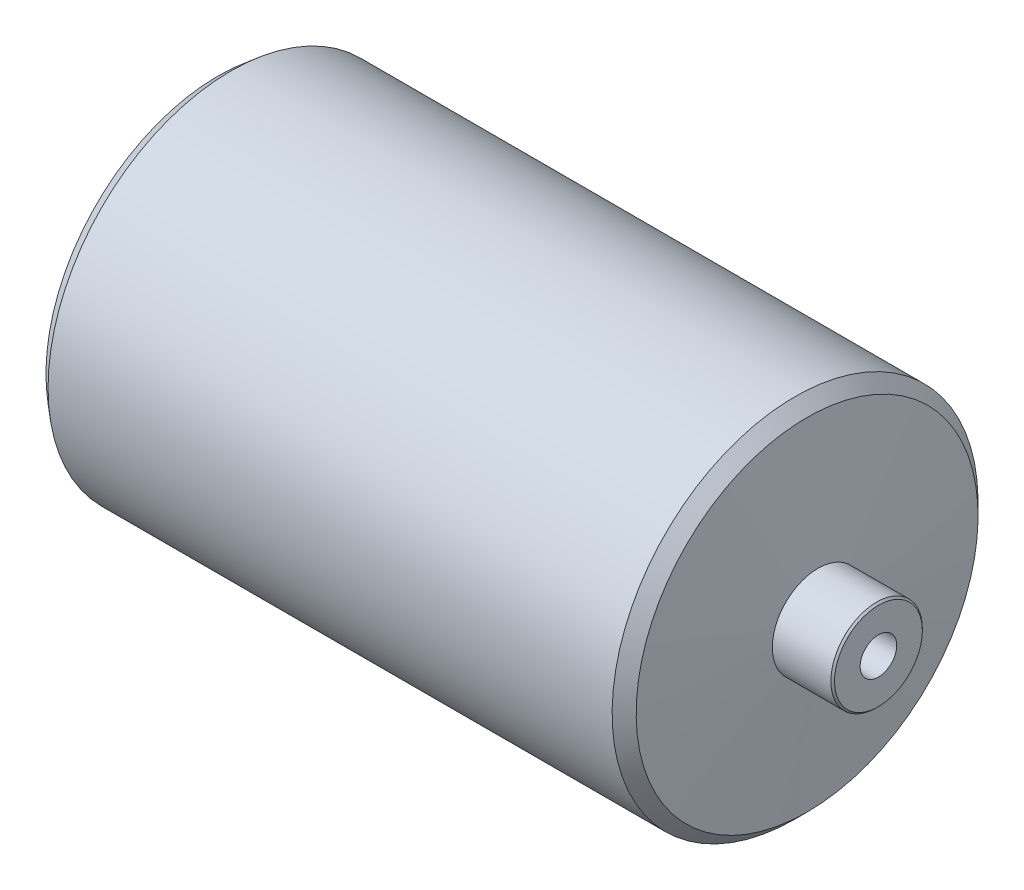
ISO-10303-21;
HEADER;
FILE_DESCRIPTION(('STEP AP214'),'2;1');
FILE_NAME('part.step','',(''),(''),'','','');
FILE_SCHEMA(('AUTOMOTIVE_DESIGN { 1 0 10303 214 1 1 1 1 }'));
ENDSEC;
DATA;
#1=APPLICATION_CONTEXT('core data for automotive mechanical design processes');
#2=APPLICATION_PROTOCOL_DEFINITION('international standard','automotive_design',2000,#1);
#3=PRODUCT_CONTEXT('',#1,'mechanical');
#4=PRODUCT('Part','Part','',(#3));
#5=PRODUCT_RELATED_PRODUCT_CATEGORY('part','',(#4));
#6=PRODUCT_DEFINITION_FORMATION('','',#4);
#7=PRODUCT_DEFINITION_CONTEXT('part definition',#1,'design');
#8=PRODUCT_DEFINITION('design','',#6,#7);
#9=PRODUCT_DEFINITION_SHAPE('','',#8);
#10=(LENGTH_UNIT() NAMED_UNIT(*) SI_UNIT(.MILLI.,.METRE.));
#11=(NAMED_UNIT(*) PLANE_ANGLE_UNIT() SI_UNIT($,.RADIAN.));
#12=(NAMED_UNIT(*) SI_UNIT($,.STERADIAN.) SOLID_ANGLE_UNIT());
#13=UNCERTAINTY_MEASURE_WITH_UNIT(LENGTH_MEASURE(1.E-05),#10,'distance_accuracy_value','');
#14=(GEOMETRIC_REPRESENTATION_CONTEXT(3) GLOBAL_UNCERTAINTY_ASSIGNED_CONTEXT((#13)) GLOBAL_UNIT_ASSIGNED_CONTEXT((#10,
#11,#12)) REPRESENTATION_CONTEXT('',''));
#15=CARTESIAN_POINT('',(0.,0.,0.));
#16=DIRECTION('',(0.,0.,1.));
#17=DIRECTION('',(1.,0.,0.));
#18=AXIS2_PLACEMENT_3D('',#15,#16,#17);
#19=CARTESIAN_POINT('',(0.,0.,0.));
#20=DIRECTION('',(-1.,0.,0.));
#21=DIRECTION('',(0.,-1.,0.));
#22=AXIS2_PLACEMENT_3D('',#19,#20,#21);
#23=PLANE('',#22);
#24=CARTESIAN_POINT('',(0.,0.,0.));
#25=DIRECTION('',(-1.,0.,0.));
#26=DIRECTION('',(0.,0.,1.));
#27=AXIS2_PLACEMENT_3D('',#24,#25,#26);
#28=CIRCLE('',#27,5.00000000000001);
#29=CARTESIAN_POINT('',(0.,0.,5.00000000000001));
#30=VERTEX_POINT('',#29);
#31=EDGE_CURVE('E90',#30,#30,#28,.T.);
#32=ORIENTED_EDGE('',*,*,#31,.F.);
#33=EDGE_LOOP('',(#32));
#34=FACE_BOUND('',#33,.T.);
#35=CARTESIAN_POINT('',(0.,0.,0.));
#36=DIRECTION('',(-1.,0.,0.));
#37=DIRECTION('',(0.,-1.,0.));
#38=AXIS2_PLACEMENT_3D('',#35,#36,#37);
#39=CIRCLE('',#38,12.);
#40=CARTESIAN_POINT('',(0.,-12.,0.));
#41=VERTEX_POINT('',#40);
#42=EDGE_CURVE('E58',#41,#41,#39,.T.);
#43=ORIENTED_EDGE('',*,*,#42,.T.);
#44=EDGE_LOOP('',(#43));
#45=FACE_BOUND('',#44,.T.);
#46=ADVANCED_FACE('F39',(#34,#45),#23,.T.);
#47=CARTESIAN_POINT('',(200.,0.,0.));
#48=DIRECTION('',(1.,0.,0.));
#49=DIRECTION('',(0.,1.,0.));
#50=AXIS2_PLACEMENT_3D('',#47,#48,#49);
#51=CYLINDRICAL_SURFACE('',#50,12.5);
#52=CARTESIAN_POINT('',(0.500000000000056,0.,0.));
#53=DIRECTION('',(-1.,0.,0.));
#54=DIRECTION('',(0.,-1.,0.));
#55=AXIS2_PLACEMENT_3D('',#52,#53,#54);
#56=CIRCLE('',#55,12.5);
#57=CARTESIAN_POINT('',(0.500000000000057,-12.5,0.));
#58=VERTEX_POINT('',#57);
#59=EDGE_CURVE('E62',#58,#58,#56,.F.);
#60=ORIENTED_EDGE('',*,*,#59,.T.);
#61=EDGE_LOOP('',(#60));
#62=FACE_BOUND('',#61,.T.);
#63=CARTESIAN_POINT('',(16.5,0.,0.));
#64=DIRECTION('',(1.,0.,0.));
#65=DIRECTION('',(0.,1.,0.));
#66=AXIS2_PLACEMENT_3D('',#63,#64,#65);
#67=CIRCLE('',#66,12.5);
#68=CARTESIAN_POINT('',(16.5,12.5,0.));
#69=VERTEX_POINT('',#68);
#70=EDGE_CURVE('E75',#69,#69,#67,.T.);
#71=ORIENTED_EDGE('',*,*,#70,.F.);
#72=EDGE_LOOP('',(#71));
#73=FACE_BOUND('',#72,.T.);
#74=ADVANCED_FACE('F94',(#62,#73),#51,.T.);
#75=CARTESIAN_POINT('',(19.7808248822223,0.,0.));
#76=DIRECTION('',(1.,0.,0.));
#77=DIRECTION('',(0.,1.,0.));
#78=AXIS2_PLACEMENT_3D('',#75,#76,#77);
#79=CONICAL_SURFACE('',#78,50.,1.48352986419518);
#80=CARTESIAN_POINT('',(19.5193576539793,0.,0.));
#81=DIRECTION('',(-1.,0.,0.));
#82=DIRECTION('',(0.,-1.,0.));
#83=AXIS2_PLACEMENT_3D('',#80,#81,#82);
#84=CIRCLE('',#83,47.0114159057247);
#85=CARTESIAN_POINT('',(19.5193576539793,47.0114159057247,0.));
#86=VERTEX_POINT('',#85);
#87=EDGE_CURVE('E50',#86,#86,#84,.T.);
#88=CARTESIAN_POINT('',(19.5193576539793,47.0114159057247,0.));
#89=CARTESIAN_POINT('',(19.4879060117504,46.6519219900401,0.));
#90=CARTESIAN_POINT('',(19.4564543695214,46.2924280743555,0.));
#91=CARTESIAN_POINT('',(19.3935510850635,45.5734402429862,0.));
#92=CARTESIAN_POINT('',(19.3620994428346,45.2139463273016,0.));
#93=CARTESIAN_POINT('',(19.2991961583767,44.4949584959323,0.));
#94=CARTESIAN_POINT('',(19.2677445161477,44.1354645802477,0.));
#95=CARTESIAN_POINT('',(19.2048412316898,43.4164767488784,0.));
#96=CARTESIAN_POINT('',(19.1733895894609,43.0569828331938,0.));
#97=CARTESIAN_POINT('',(19.1104863050029,42.3379950018245,0.));
#98=CARTESIAN_POINT('',(19.079034662774,41.9785010861399,0.));
#99=CARTESIAN_POINT('',(19.0161313783161,41.2595132547706,0.));
#100=CARTESIAN_POINT('',(18.9846797360871,40.900019339086,0.));
#101=CARTESIAN_POINT('',(18.9217764516292,40.1810315077167,0.));
#102=CARTESIAN_POINT('',(18.8903248094003,39.8215375920321,0.));
#103=CARTESIAN_POINT('',(18.8274215249424,39.1025497606628,0.));
#104=CARTESIAN_POINT('',(18.7959698827134,38.7430558449782,0.));
#105=CARTESIAN_POINT('',(18.7330665982555,38.0240680136089,0.));
#106=CARTESIAN_POINT('',(18.7016149560266,37.6645740979243,0.));
#107=CARTESIAN_POINT('',(18.6387116715687,36.945586266555,0.));
#108=CARTESIAN_POINT('',(18.6072600293397,36.5860923508704,0.));
#109=CARTESIAN_POINT('',(18.5443567448818,35.8671045195011,0.));
#110=CARTESIAN_POINT('',(18.5129051026529,35.5076106038165,0.));
#111=CARTESIAN_POINT('',(18.450001818195,34.7886227724472,0.));
#112=CARTESIAN_POINT('',(18.418550175966,34.4291288567626,0.));
#113=CARTESIAN_POINT('',(18.3556468915081,33.7101410253933,0.));
#114=CARTESIAN_POINT('',(18.3241952492792,33.3506471097087,0.));
#115=CARTESIAN_POINT('',(18.2612919648213,32.6316592783394,0.));
#116=CARTESIAN_POINT('',(18.2298403225923,32.2721653626548,0.));
#117=CARTESIAN_POINT('',(18.1669370381344,31.5531775312855,0.));
#118=CARTESIAN_POINT('',(18.1354853959055,31.1936836156009,0.));
#119=CARTESIAN_POINT('',(18.0725821114476,30.4746957842316,0.));
#120=CARTESIAN_POINT('',(18.0411304692186,30.115201868547,0.));
#121=CARTESIAN_POINT('',(17.9782271847607,29.3962140371777,0.));
#122=CARTESIAN_POINT('',(17.9467755425318,29.0367201214931,0.));
#123=CARTESIAN_POINT('',(17.8838722580739,28.3177322901238,0.));
#124=CARTESIAN_POINT('',(17.8524206158449,27.9582383744392,0.));
#125=CARTESIAN_POINT('',(17.789517331387,27.2392505430699,0.));
#126=CARTESIAN_POINT('',(17.7580656891581,26.8797566273853,0.));
#127=CARTESIAN_POINT('',(17.6951624047002,26.160768796016,0.));
#128=CARTESIAN_POINT('',(17.6637107624712,25.8012748803314,0.));
#129=CARTESIAN_POINT('',(17.6008074780133,25.0822870489621,0.));
#130=CARTESIAN_POINT('',(17.5693558357844,24.7227931332775,0.));
#131=CARTESIAN_POINT('',(17.5064525513264,24.0038053019082,0.));
#132=CARTESIAN_POINT('',(17.4750009090975,23.6443113862236,0.));
#133=CARTESIAN_POINT('',(17.4120976246396,22.9253235548543,0.));
#134=CARTESIAN_POINT('',(17.3806459824106,22.5658296391697,0.));
#135=CARTESIAN_POINT('',(17.3177426979527,21.8468418078004,0.));
#136=CARTESIAN_POINT('',(17.2862910557238,21.4873478921158,0.));
#137=CARTESIAN_POINT('',(17.2233877712659,20.7683600607465,0.));
#138=CARTESIAN_POINT('',(17.1919361290369,20.4088661450619,0.));
#139=CARTESIAN_POINT('',(17.129032844579,19.6898783136926,0.));
#140=CARTESIAN_POINT('',(17.0975812023501,19.330384398008,0.));
#141=CARTESIAN_POINT('',(17.0346779178922,18.6113965666387,0.));
#142=CARTESIAN_POINT('',(17.0032262756632,18.2519026509541,0.));
#143=CARTESIAN_POINT('',(16.9403229912053,17.5329148195848,0.));
#144=CARTESIAN_POINT('',(16.9088713489764,17.1734209039002,0.));
#145=CARTESIAN_POINT('',(16.8459680645185,16.4544330725309,0.));
#146=CARTESIAN_POINT('',(16.8145164222895,16.0949391568463,0.));
#147=CARTESIAN_POINT('',(16.7516131378316,15.375951325477,0.));
#148=CARTESIAN_POINT('',(16.7201614956027,15.0164574097924,0.));
#149=CARTESIAN_POINT('',(16.6572582111448,14.2974695784231,0.));
#150=CARTESIAN_POINT('',(16.6258065689158,13.9379756627385,0.));
#151=CARTESIAN_POINT('',(16.5629032844579,13.2189878313692,0.));
#152=CARTESIAN_POINT('',(16.531451642229,12.8594939156846,0.));
#153=CARTESIAN_POINT('',(16.5,12.5,0.));
#154=B_SPLINE_CURVE_WITH_KNOTS('',3,(#88,#89,#90,#91,#92,#93,#94,#95,#96,#97,#98,#99,#100,#101,
#102,#103,#104,#105,#106,#107,#108,#109,#110,#111,#112,#113,#114,#115,#116,#117,#118,#119,#120,
#121,#122,#123,#124,#125,#126,#127,#128,#129,#130,#131,#132,#133,#134,#135,#136,#137,#138,#139,
#140,#141,#142,#143,#144,#145,#146,#147,#148,#149,#150,#151,#152,#153),.UNSPECIFIED.,.F.,.F.,(4,
2,2,2,2,2,2,2,2,2,2,2,2,2,2,2,2,2,2,2,2,2,2,2,2,2,2,2,2,2,2,2,4),(0.,1.08260137212111,
2.16520274424222,3.24780411636333,4.33040548848443,5.41300686060555,6.49560823272666,
7.57820960484777,8.66081097696888,9.74341234908999,10.8260137212111,11.9086150933322,
12.9912164654533,14.0738178375744,15.1564192096955,16.2390205818167,17.3216219539378,
18.4042233260589,19.48682469818,20.5694260703011,21.6520274424222,22.7346288145433,
23.8172301866644,24.8998315587855,25.9824329309067,27.0650343030278,28.1476356751489,
29.23023704727,30.3128384193911,31.3954397915122,32.4780411636333,33.5606425357544,
34.6432439078755),.UNSPECIFIED.);
#155=EDGE_CURVE('BSEAM107',#86,#69,#154,.T.);
#156=ORIENTED_EDGE('',*,*,#87,.T.);
#157=ORIENTED_EDGE('',*,*,#70,.T.);
#158=ORIENTED_EDGE('',*,*,#155,.T.);
#159=ORIENTED_EDGE('',*,*,#155,.F.);
#160=EDGE_LOOP('',(#156,#158,#157,#159));
#161=FACE_BOUND('',#160,.T.);
#162=ADVANCED_FACE('F107',(#161),#79,.T.);
#163=CARTESIAN_POINT('',(200.,0.,0.));
#164=DIRECTION('',(1.,0.,0.));
#165=DIRECTION('',(0.,1.,0.));
#166=AXIS2_PLACEMENT_3D('',#163,#164,#165);
#167=CYLINDRICAL_SURFACE('',#166,50.);
#168=CARTESIAN_POINT('',(23.0810134851018,0.,0.));
#169=DIRECTION('',(-1.,0.,0.));
#170=DIRECTION('',(0.,-1.,0.));
#171=AXIS2_PLACEMENT_3D('',#168,#169,#170);
#172=CIRCLE('',#171,50.);
#173=CARTESIAN_POINT('',(23.0810134851018,-50.,0.));
#174=VERTEX_POINT('',#173);
#175=EDGE_CURVE('E51',#174,#174,#172,.F.);
#176=ORIENTED_EDGE('',*,*,#175,.T.);
#177=EDGE_LOOP('',(#176));
#178=FACE_BOUND('',#177,.T.);
#179=CARTESIAN_POINT('',(177.219175117778,0.,0.));
#180=DIRECTION('',(1.,0.,0.));
#181=DIRECTION('',(0.,1.,0.));
#182=AXIS2_PLACEMENT_3D('',#179,#180,#181);
#183=CIRCLE('',#182,50.);
#184=CARTESIAN_POINT('',(177.219175117778,-50.,0.));
#185=VERTEX_POINT('',#184);
#186=EDGE_CURVE('E54',#185,#185,#183,.F.);
#187=ORIENTED_EDGE('',*,*,#186,.T.);
#188=EDGE_LOOP('',(#187));
#189=FACE_BOUND('',#188,.T.);
#190=ADVANCED_FACE('F112',(#178,#189),#167,.T.);
#191=CARTESIAN_POINT('',(183.5,0.,0.));
#192=DIRECTION('',(-1.,0.,0.));
#193=DIRECTION('',(0.,-1.,0.));
#194=AXIS2_PLACEMENT_3D('',#191,#192,#193);
#195=CONICAL_SURFACE('',#194,12.5,1.48352986419518);
#196=CARTESIAN_POINT('',(180.506805506669,0.,0.));
#197=DIRECTION('',(1.,0.,0.));
#198=DIRECTION('',(0.,1.,0.));
#199=AXIS2_PLACEMENT_3D('',#196,#197,#198);
#200=CIRCLE('',#199,46.7123696111087);
#201=CARTESIAN_POINT('',(180.506805506669,-46.7123696111086,0.));
#202=VERTEX_POINT('',#201);
#203=EDGE_CURVE('E10',#202,#202,#200,.T.);
#204=CARTESIAN_POINT('',(183.5,0.,0.));
#205=DIRECTION('',(1.,0.,0.));
#206=DIRECTION('',(0.,1.,0.));
#207=AXIS2_PLACEMENT_3D('',#204,#205,#206);
#208=CIRCLE('',#207,12.5);
#209=CARTESIAN_POINT('',(183.5,-12.4999999999998,0.));
#210=VERTEX_POINT('',#209);
#211=EDGE_CURVE('E74',#210,#210,#208,.T.);
#212=CARTESIAN_POINT('',(180.506805506669,-46.7123696111086,0.));
#213=CARTESIAN_POINT('',(180.537984615975,-46.3559907609929,0.));
#214=CARTESIAN_POINT('',(180.56916372528,-45.9996119108772,0.));
#215=CARTESIAN_POINT('',(180.631521943891,-45.2868542106457,0.));
#216=CARTESIAN_POINT('',(180.662701053197,-44.93047536053,0.));
#217=CARTESIAN_POINT('',(180.725059271808,-44.2177176602986,0.));
#218=CARTESIAN_POINT('',(180.756238381113,-43.8613388101829,0.));
#219=CARTESIAN_POINT('',(180.818596599724,-43.1485811099514,0.));
#220=CARTESIAN_POINT('',(180.84977570903,-42.7922022598357,0.));
#221=CARTESIAN_POINT('',(180.912133927641,-42.0794445596043,0.));
#222=CARTESIAN_POINT('',(180.943313036946,-41.7230657094886,0.));
#223=CARTESIAN_POINT('',(181.005671255558,-41.0103080092571,0.));
#224=CARTESIAN_POINT('',(181.036850364863,-40.6539291591414,0.));
#225=CARTESIAN_POINT('',(181.099208583474,-39.94117145891,0.));
#226=CARTESIAN_POINT('',(181.13038769278,-39.5847926087943,0.));
#227=CARTESIAN_POINT('',(181.192745911391,-38.8720349085628,0.));
#228=CARTESIAN_POINT('',(181.223925020696,-38.5156560584471,0.));
#229=CARTESIAN_POINT('',(181.286283239307,-37.8028983582157,0.));
#230=CARTESIAN_POINT('',(181.317462348613,-37.4465195081,0.));
#231=CARTESIAN_POINT('',(181.379820567224,-36.7337618078685,0.));
#232=CARTESIAN_POINT('',(181.410999676529,-36.3773829577528,0.));
#233=CARTESIAN_POINT('',(181.47335789514,-35.6646252575214,0.));
#234=CARTESIAN_POINT('',(181.504537004446,-35.3082464074057,0.));
#235=CARTESIAN_POINT('',(181.566895223057,-34.5954887071742,0.));
#236=CARTESIAN_POINT('',(181.598074332363,-34.2391098570585,0.));
#237=CARTESIAN_POINT('',(181.660432550974,-33.5263521568271,0.));
#238=CARTESIAN_POINT('',(181.691611660279,-33.1699733067114,0.));
#239=CARTESIAN_POINT('',(181.75396987889,-32.4572156064799,0.));
#240=CARTESIAN_POINT('',(181.785148988196,-32.1008367563642,0.));
#241=CARTESIAN_POINT('',(181.847507206807,-31.3880790561328,0.));
#242=CARTESIAN_POINT('',(181.878686316112,-31.0317002060171,0.));
#243=CARTESIAN_POINT('',(181.941044534723,-30.3189425057856,0.));
#244=CARTESIAN_POINT('',(181.972223644029,-29.9625636556699,0.));
#245=CARTESIAN_POINT('',(182.03458186264,-29.2498059554385,0.));
#246=CARTESIAN_POINT('',(182.065760971946,-28.8934271053228,0.));
#247=CARTESIAN_POINT('',(182.128119190557,-28.1806694050913,0.));
#248=CARTESIAN_POINT('',(182.159298299862,-27.8242905549756,0.));
#249=CARTESIAN_POINT('',(182.221656518473,-27.1115328547442,0.));
#250=CARTESIAN_POINT('',(182.252835627779,-26.7551540046285,0.));
#251=CARTESIAN_POINT('',(182.31519384639,-26.042396304397,0.));
#252=CARTESIAN_POINT('',(182.346372955695,-25.6860174542813,0.));
#253=CARTESIAN_POINT('',(182.408731174306,-24.9732597540499,0.));
#254=CARTESIAN_POINT('',(182.439910283612,-24.6168809039342,0.));
#255=CARTESIAN_POINT('',(182.502268502223,-23.9041232037028,0.));
#256=CARTESIAN_POINT('',(182.533447611529,-23.547744353587,0.));
#257=CARTESIAN_POINT('',(182.59580583014,-22.8349866533556,0.));
#258=CARTESIAN_POINT('',(182.626984939445,-22.4786078032399,0.));
#259=CARTESIAN_POINT('',(182.689343158056,-21.7658501030085,0.));
#260=CARTESIAN_POINT('',(182.720522267362,-21.4094712528927,0.));
#261=CARTESIAN_POINT('',(182.782880485973,-20.6967135526613,0.));
#262=CARTESIAN_POINT('',(182.814059595278,-20.3403347025456,0.));
#263=CARTESIAN_POINT('',(182.876417813889,-19.6275770023142,0.));
#264=CARTESIAN_POINT('',(182.907596923195,-19.2711981521984,0.));
#265=CARTESIAN_POINT('',(182.969955141806,-18.558440451967,0.));
#266=CARTESIAN_POINT('',(183.001134251112,-18.2020616018513,0.));
#267=CARTESIAN_POINT('',(183.063492469723,-17.4893039016199,0.));
#268=CARTESIAN_POINT('',(183.094671579028,-17.1329250515041,0.));
#269=CARTESIAN_POINT('',(183.157029797639,-16.4201673512727,0.));
#270=CARTESIAN_POINT('',(183.188208906945,-16.063788501157,0.));
#271=CARTESIAN_POINT('',(183.250567125556,-15.3510308009256,0.));
#272=CARTESIAN_POINT('',(183.281746234861,-14.9946519508098,0.));
#273=CARTESIAN_POINT('',(183.344104453472,-14.2818942505784,0.));
#274=CARTESIAN_POINT('',(183.375283562778,-13.9255154004627,0.));
#275=CARTESIAN_POINT('',(183.437641781389,-13.2127577002313,0.));
#276=CARTESIAN_POINT('',(183.468820890694,-12.8563788501155,0.));
#277=CARTESIAN_POINT('',(183.5,-12.4999999999998,0.));
#278=B_SPLINE_CURVE_WITH_KNOTS('',3,(#212,#213,#214,#215,#216,#217,#218,#219,#220,#221,#222,
#223,#224,#225,#226,#227,#228,#229,#230,#231,#232,#233,#234,#235,#236,#237,#238,#239,#240,#241,
#242,#243,#244,#245,#246,#247,#248,#249,#250,#251,#252,#253,#254,#255,#256,#257,#258,#259,#260,
#261,#262,#263,#264,#265,#266,#267,#268,#269,#270,#271,#272,#273,#274,#275,#276,#277),
.UNSPECIFIED.,.F.,.F.,(4,2,2,2,2,2,2,2,2,2,2,2,2,2,2,2,2,2,2,2,2,2,2,2,2,2,2,2,2,2,2,2,4),(0.,
1.07322047828112,2.14644095656226,3.21966143484338,4.29288191312452,5.36610239140565,
6.43932286968678,7.51254334796791,8.58576382624904,9.65898430453017,10.7322047828113,
11.8054252610924,12.8786457393736,13.9518662176547,15.0250866959358,16.0983071742169,
17.1715276524981,18.2447481307792,19.3179686090603,20.3911890873415,21.4644095656226,
22.5376300439037,23.6108505221849,24.684071000466,25.7572914787471,26.8305119570283,
27.9037324353094,28.9769529135905,30.0501733918717,31.1233938701528,32.1966143484339,
33.269834826715,34.3430553049962),.UNSPECIFIED.);
#279=EDGE_CURVE('BSEAM118',#202,#210,#278,.T.);
#280=ORIENTED_EDGE('',*,*,#203,.T.);
#281=ORIENTED_EDGE('',*,*,#211,.F.);
#282=ORIENTED_EDGE('',*,*,#279,.T.);
#283=ORIENTED_EDGE('',*,*,#279,.F.);
#284=EDGE_LOOP('',(#280,#282,#281,#283));
#285=FACE_BOUND('',#284,.T.);
#286=ADVANCED_FACE('F118',(#285),#195,.T.);
#287=CARTESIAN_POINT('',(200.,0.,0.));
#288=DIRECTION('',(1.,0.,0.));
#289=DIRECTION('',(0.,1.,0.));
#290=AXIS2_PLACEMENT_3D('',#287,#288,#289);
#291=CYLINDRICAL_SURFACE('',#290,12.5);
#292=CARTESIAN_POINT('',(199.5,0.,0.));
#293=DIRECTION('',(1.,0.,0.));
#294=DIRECTION('',(0.,1.,0.));
#295=AXIS2_PLACEMENT_3D('',#292,#293,#294);
#296=CIRCLE('',#295,12.5);
#297=CARTESIAN_POINT('',(199.5,12.5,0.));
#298=VERTEX_POINT('',#297);
#299=EDGE_CURVE('E66',#298,#298,#296,.F.);
#300=ORIENTED_EDGE('',*,*,#299,.T.);
#301=EDGE_LOOP('',(#300));
#302=FACE_BOUND('',#301,.T.);
#303=ORIENTED_EDGE('',*,*,#211,.T.);
#304=EDGE_LOOP('',(#303));
#305=FACE_BOUND('',#304,.T.);
#306=ADVANCED_FACE('F164',(#302,#305),#291,.T.);
#307=CARTESIAN_POINT('',(200.,12.5,0.));
#308=DIRECTION('',(1.,0.,0.));
#309=DIRECTION('',(0.,1.,0.));
#310=AXIS2_PLACEMENT_3D('',#307,#308,#309);
#311=PLANE('',#310);
#312=CARTESIAN_POINT('',(200.,0.,0.));
#313=DIRECTION('',(1.,0.,0.));
#314=DIRECTION('',(0.,0.,-1.));
#315=AXIS2_PLACEMENT_3D('',#312,#313,#314);
#316=CIRCLE('',#315,5.00000000000001);
#317=CARTESIAN_POINT('',(200.,0.,-5.00000000000001));
#318=VERTEX_POINT('',#317);
#319=EDGE_CURVE('E81',#318,#318,#316,.T.);
#320=ORIENTED_EDGE('',*,*,#319,.F.);
#321=EDGE_LOOP('',(#320));
#322=FACE_BOUND('',#321,.T.);
#323=CARTESIAN_POINT('',(200.,0.,0.));
#324=DIRECTION('',(1.,0.,0.));
#325=DIRECTION('',(0.,1.,0.));
#326=AXIS2_PLACEMENT_3D('',#323,#324,#325);
#327=CIRCLE('',#326,12.);
#328=CARTESIAN_POINT('',(200.,12.,0.));
#329=VERTEX_POINT('',#328);
#330=EDGE_CURVE('E68',#329,#329,#327,.T.);
#331=ORIENTED_EDGE('',*,*,#330,.T.);
#332=EDGE_LOOP('',(#331));
#333=FACE_BOUND('',#332,.T.);
#334=ADVANCED_FACE('F128',(#322,#333),#311,.T.);
#335=CARTESIAN_POINT('',(200.,0.,0.));
#336=DIRECTION('',(-1.,0.,0.));
#337=DIRECTION('',(0.,-1.,0.));
#338=AXIS2_PLACEMENT_3D('',#335,#336,#337);
#339=CONICAL_SURFACE('',#338,12.,0.785398163397431);
#340=ORIENTED_EDGE('',*,*,#299,.F.);
#341=EDGE_LOOP('',(#340));
#342=FACE_BOUND('',#341,.T.);
#343=ORIENTED_EDGE('',*,*,#330,.F.);
#344=EDGE_LOOP('',(#343));
#345=FACE_BOUND('',#344,.T.);
#346=ADVANCED_FACE('F101',(#342,#345),#339,.T.);
#347=CARTESIAN_POINT('',(0.500000000000056,0.,0.));
#348=DIRECTION('',(1.,0.,0.));
#349=DIRECTION('',(0.,1.,0.));
#350=AXIS2_PLACEMENT_3D('',#347,#348,#349);
#351=CONICAL_SURFACE('',#350,12.5,0.785398163397438);
#352=ORIENTED_EDGE('',*,*,#42,.F.);
#353=EDGE_LOOP('',(#352));
#354=FACE_BOUND('',#353,.T.);
#355=ORIENTED_EDGE('',*,*,#59,.F.);
#356=EDGE_LOOP('',(#355));
#357=FACE_BOUND('',#356,.T.);
#358=ADVANCED_FACE('F100',(#354,#357),#351,.T.);
#359=CARTESIAN_POINT('',(23.0810134851018,0.,0.));
#360=DIRECTION('',(1.,0.,0.));
#361=DIRECTION('',(0.,1.,0.));
#362=AXIS2_PLACEMENT_3D('',#359,#360,#361);
#363=CONICAL_SURFACE('',#362,50.,0.698131700797729);
#364=ORIENTED_EDGE('',*,*,#87,.F.);
#365=EDGE_LOOP('',(#364));
#366=FACE_BOUND('',#365,.T.);
#367=ORIENTED_EDGE('',*,*,#175,.F.);
#368=EDGE_LOOP('',(#367));
#369=FACE_BOUND('',#368,.T.);
#370=ADVANCED_FACE('F105',(#366,#369),#363,.T.);
#371=CARTESIAN_POINT('',(180.506805506669,0.,0.));
#372=DIRECTION('',(-1.,0.,0.));
#373=DIRECTION('',(0.,-1.,0.));
#374=AXIS2_PLACEMENT_3D('',#371,#372,#373);
#375=CONICAL_SURFACE('',#374,46.7123696111087,0.785398163397439);
#376=CARTESIAN_POINT('',(177.219175117778,-50.,0.));
#377=CARTESIAN_POINT('',(177.253421267662,-49.9657538501157,0.));
#378=CARTESIAN_POINT('',(177.287667417546,-49.9315077002314,0.));
#379=CARTESIAN_POINT('',(177.356159717315,-49.8630154004628,0.));
#380=CARTESIAN_POINT('',(177.390405867199,-49.8287692505785,0.));
#381=CARTESIAN_POINT('',(177.458898166968,-49.76027695081,0.));
#382=CARTESIAN_POINT('',(177.493144316852,-49.7260308009257,0.));
#383=CARTESIAN_POINT('',(177.561636616621,-49.6575385011571,0.));
#384=CARTESIAN_POINT('',(177.595882766505,-49.6232923512728,0.));
#385=CARTESIAN_POINT('',(177.664375066273,-49.5548000515043,0.));
#386=CARTESIAN_POINT('',(177.698621216158,-49.52055390162,0.));
#387=CARTESIAN_POINT('',(177.767113515926,-49.4520616018514,0.));
#388=CARTESIAN_POINT('',(177.801359665811,-49.4178154519671,0.));
#389=CARTESIAN_POINT('',(177.869851965579,-49.3493231521986,0.));
#390=CARTESIAN_POINT('',(177.904098115463,-49.3150770023143,0.));
#391=CARTESIAN_POINT('',(177.972590415232,-49.2465847025457,0.));
#392=CARTESIAN_POINT('',(178.006836565116,-49.2123385526614,0.));
#393=CARTESIAN_POINT('',(178.075328864885,-49.1438462528928,0.));
#394=CARTESIAN_POINT('',(178.109575014769,-49.1096001030086,0.));
#395=CARTESIAN_POINT('',(178.178067314538,-49.04110780324,0.));
#396=CARTESIAN_POINT('',(178.212313464422,-49.0068616533557,0.));
#397=CARTESIAN_POINT('',(178.280805764191,-48.9383693535871,0.));
#398=CARTESIAN_POINT('',(178.315051914075,-48.9041232037029,0.));
#399=CARTESIAN_POINT('',(178.383544213843,-48.8356309039343,0.));
#400=CARTESIAN_POINT('',(178.417790363728,-48.80138475405,0.));
#401=CARTESIAN_POINT('',(178.486282663496,-48.7328924542814,0.));
#402=CARTESIAN_POINT('',(178.520528813381,-48.6986463043972,0.));
#403=CARTESIAN_POINT('',(178.589021113149,-48.6301540046286,0.));
#404=CARTESIAN_POINT('',(178.623267263033,-48.5959078547443,0.));
#405=CARTESIAN_POINT('',(178.691759562802,-48.5274155549757,0.));
#406=CARTESIAN_POINT('',(178.726005712686,-48.4931694050914,0.));
#407=CARTESIAN_POINT('',(178.794498012455,-48.4246771053229,0.));
#408=CARTESIAN_POINT('',(178.828744162339,-48.3904309554386,0.));
#409=CARTESIAN_POINT('',(178.897236462108,-48.32193865567,0.));
#410=CARTESIAN_POINT('',(178.931482611992,-48.2876925057857,0.));
#411=CARTESIAN_POINT('',(178.999974911761,-48.2192002060172,0.));
#412=CARTESIAN_POINT('',(179.034221061645,-48.1849540561329,0.));
#413=CARTESIAN_POINT('',(179.102713361413,-48.1164617563643,0.));
#414=CARTESIAN_POINT('',(179.136959511298,-48.08221560648,0.));
#415=CARTESIAN_POINT('',(179.205451811066,-48.0137233067115,0.));
#416=CARTESIAN_POINT('',(179.239697960951,-47.9794771568272,0.));
#417=CARTESIAN_POINT('',(179.308190260719,-47.9109848570586,0.));
#418=CARTESIAN_POINT('',(179.342436410603,-47.8767387071743,0.));
#419=CARTESIAN_POINT('',(179.410928710372,-47.8082464074058,0.));
#420=CARTESIAN_POINT('',(179.445174860256,-47.7740002575215,0.));
#421=CARTESIAN_POINT('',(179.513667160025,-47.7055079577529,0.));
#422=CARTESIAN_POINT('',(179.547913309909,-47.6712618078686,0.));
#423=CARTESIAN_POINT('',(179.616405609678,-47.6027695081001,0.));
#424=CARTESIAN_POINT('',(179.650651759562,-47.5685233582158,0.));
#425=CARTESIAN_POINT('',(179.719144059331,-47.5000310584472,0.));
#426=CARTESIAN_POINT('',(179.753390209215,-47.4657849085629,0.));
#427=CARTESIAN_POINT('',(179.821882508983,-47.3972926087944,0.));
#428=CARTESIAN_POINT('',(179.856128658868,-47.3630464589101,0.));
#429=CARTESIAN_POINT('',(179.924620958636,-47.2945541591415,0.));
#430=CARTESIAN_POINT('',(179.95886710852,-47.2603080092572,0.));
#431=CARTESIAN_POINT('',(180.027359408289,-47.1918157094887,0.));
#432=CARTESIAN_POINT('',(180.061605558173,-47.1575695596044,0.));
#433=CARTESIAN_POINT('',(180.130097857942,-47.0890772598358,0.));
#434=CARTESIAN_POINT('',(180.164344007826,-47.0548311099515,0.));
#435=CARTESIAN_POINT('',(180.232836307595,-46.9863388101829,0.));
#436=CARTESIAN_POINT('',(180.267082457479,-46.9520926602986,0.));
#437=CARTESIAN_POINT('',(180.335574757248,-46.8836003605301,0.));
#438=CARTESIAN_POINT('',(180.369820907132,-46.8493542106458,0.));
#439=CARTESIAN_POINT('',(180.4383132069,-46.7808619108772,0.));
#440=CARTESIAN_POINT('',(180.472559356785,-46.746615760993,0.));
#441=CARTESIAN_POINT('',(180.506805506669,-46.7123696111087,0.));
#442=B_SPLINE_CURVE_WITH_KNOTS('',3,(#376,#377,#378,#379,#380,#381,#382,#383,#384,#385,#386,
#387,#388,#389,#390,#391,#392,#393,#394,#395,#396,#397,#398,#399,#400,#401,#402,#403,#404,#405,
#406,#407,#408,#409,#410,#411,#412,#413,#414,#415,#416,#417,#418,#419,#420,#421,#422,#423,#424,
#425,#426,#427,#428,#429,#430,#431,#432,#433,#434,#435,#436,#437,#438,#439,#440,#441),
.UNSPECIFIED.,.F.,.F.,(4,2,2,2,2,2,2,2,2,2,2,2,2,2,2,2,2,2,2,2,2,2,2,2,2,2,2,2,2,2,2,2,4),(0.,
0.145294108876238,0.29058821775249,0.435882326628748,0.581176435505005,0.726470544381243,
0.871764653257495,1.01705876213375,1.16235287101001,1.30764697988624,1.4529410887625,
1.59823519763876,1.74352930651502,1.88882341539125,2.03411752426751,2.17941163314376,
2.32470574202002,2.46999985089625,2.61529395977251,2.76058806864877,2.90588217752502,
3.05117628640126,3.19647039527751,3.34176450415377,3.48705861303002,3.63235272190626,
3.77764683078252,3.92294093965877,4.06823504853503,4.21352915741127,4.35882326628752,
4.50411737516378,4.64941148404001),.UNSPECIFIED.);
#443=EDGE_CURVE('BSEAM45',#185,#202,#442,.T.);
#444=ORIENTED_EDGE('',*,*,#186,.F.);
#445=ORIENTED_EDGE('',*,*,#203,.F.);
#446=ORIENTED_EDGE('',*,*,#443,.T.);
#447=ORIENTED_EDGE('',*,*,#443,.F.);
#448=EDGE_LOOP('',(#444,#446,#445,#447));
#449=FACE_BOUND('',#448,.T.);
#450=ADVANCED_FACE('F45',(#449),#375,.T.);
#451=CARTESIAN_POINT('',(141.,0.,0.));
#452=DIRECTION('',(-1.,0.,0.));
#453=DIRECTION('',(0.,0.,1.));
#454=AXIS2_PLACEMENT_3D('',#451,#452,#453);
#455=PLANE('',#454);
#456=CARTESIAN_POINT('',(141.,0.,0.));
#457=DIRECTION('',(1.,0.,0.));
#458=DIRECTION('',(0.,0.,-1.));
#459=AXIS2_PLACEMENT_3D('',#456,#457,#458);
#460=CIRCLE('',#459,5.00000000000001);
#461=CARTESIAN_POINT('',(141.,0.,-5.00000000000001));
#462=VERTEX_POINT('',#461);
#463=EDGE_CURVE('E76',#462,#462,#460,.T.);
#464=ORIENTED_EDGE('',*,*,#463,.T.);
#465=EDGE_LOOP('',(#464));
#466=FACE_BOUND('',#465,.T.);
#467=ADVANCED_FACE('F145',(#466),#455,.F.);
#468=CARTESIAN_POINT('',(200.,0.,0.));
#469=DIRECTION('',(1.,0.,0.));
#470=DIRECTION('',(0.,0.,-1.));
#471=AXIS2_PLACEMENT_3D('',#468,#469,#470);
#472=CYLINDRICAL_SURFACE('',#471,5.00000000000001);
#473=ORIENTED_EDGE('',*,*,#463,.F.);
#474=EDGE_LOOP('',(#473));
#475=FACE_BOUND('',#474,.T.);
#476=ORIENTED_EDGE('',*,*,#319,.T.);
#477=EDGE_LOOP('',(#476));
#478=FACE_BOUND('',#477,.T.);
#479=ADVANCED_FACE('F152',(#475,#478),#472,.F.);
#480=CARTESIAN_POINT('',(59.,0.,0.));
#481=DIRECTION('',(1.,0.,0.));
#482=DIRECTION('',(0.,0.,-1.));
#483=AXIS2_PLACEMENT_3D('',#480,#481,#482);
#484=PLANE('',#483);
#485=CARTESIAN_POINT('',(59.,0.,0.));
#486=DIRECTION('',(-1.,0.,0.));
#487=DIRECTION('',(0.,0.,1.));
#488=AXIS2_PLACEMENT_3D('',#485,#486,#487);
#489=CIRCLE('',#488,5.00000000000001);
#490=CARTESIAN_POINT('',(59.,0.,5.00000000000001));
#491=VERTEX_POINT('',#490);
#492=EDGE_CURVE('E83',#491,#491,#489,.T.);
#493=ORIENTED_EDGE('',*,*,#492,.T.);
#494=EDGE_LOOP('',(#493));
#495=FACE_BOUND('',#494,.T.);
#496=ADVANCED_FACE('F158',(#495),#484,.F.);
#497=CARTESIAN_POINT('',(0.,0.,0.));
#498=DIRECTION('',(-1.,0.,0.));
#499=DIRECTION('',(0.,0.,1.));
#500=AXIS2_PLACEMENT_3D('',#497,#498,#499);
#501=CYLINDRICAL_SURFACE('',#500,5.00000000000001);
#502=ORIENTED_EDGE('',*,*,#492,.F.);
#503=EDGE_LOOP('',(#502));
#504=FACE_BOUND('',#503,.T.);
#505=ORIENTED_EDGE('',*,*,#31,.T.);
#506=EDGE_LOOP('',(#505));
#507=FACE_BOUND('',#506,.T.);
#508=ADVANCED_FACE('F91',(#504,#507),#501,.F.);
#509=CLOSED_SHELL('',(#46,#74,#162,#190,#286,#306,#334,#346,#358,#370,#450,#467,#479,#496,#508));
#510=MANIFOLD_SOLID_BREP('B2',#509);
#511=ADVANCED_BREP_SHAPE_REPRESENTATION('',(#18,#510),#14);
#512=SHAPE_DEFINITION_REPRESENTATION(#9,#511);
ENDSEC;
END-ISO-10303-21;
